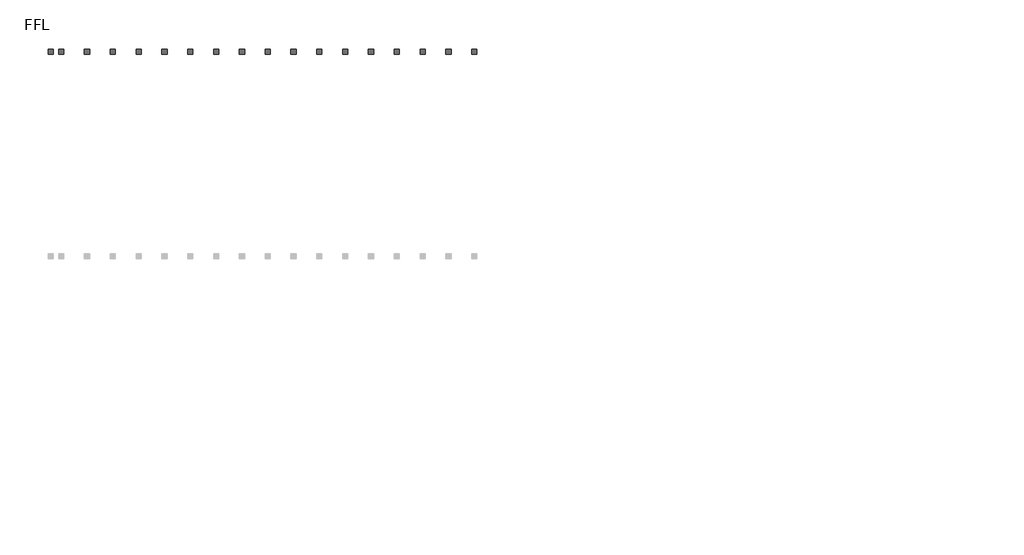
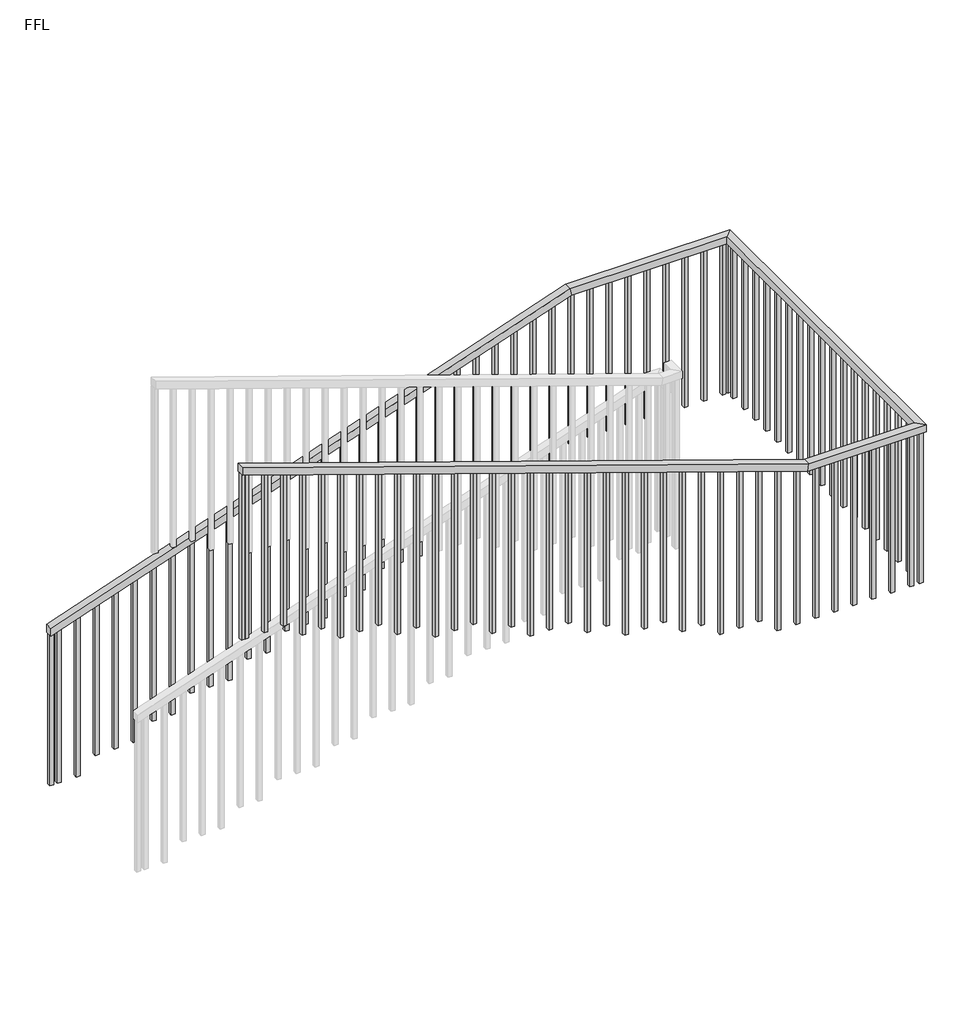
# One storey, part 2 of 2: 1 railing.
"""IFC4 building model written with IfcOpenShell, lengths in millimetres."""

from ifc_helpers import new_model, si_unit, frame, origin, place, context, project, spatial, polyline, outline, extrude, faceted_brep, element, save

model = new_model("IFC4")

# Units and contexts
model_context = context("Model", 3, world=origin())
ifc_project = project(units=[si_unit("LENGTHUNIT", "METRE", prefix="MILLI")], contexts=[model_context])

# Site, building, storey
site = spatial("IfcSite", under=ifc_project)
building = spatial("IfcBuilding", under=site)
storey = spatial("IfcBuildingStorey", under=building, Name="FFL", Elevation=3000.0)

# Railing
placement = place(None, origin())
element("IfcRailing", 1, ObjectType="1100mm", at=placement, inside=storey, context=model_context, shape_type="SolidModel", body=[
    faceted_brep([(-40149.9681829, 17835.7234223, 4656.2088216), (-40149.9681829, 17835.7234223, 4603.3636913), (-40149.9681829, 17785.7234223, 4603.3636913), (-40149.9681829, 17785.7234223, 4656.2088216), (-36733.6681829, 17835.7234223, 5824.9785156), (-36725.3519007, 17835.7234223, 5774.9785156), (-36725.3519007, 17785.7234223, 5774.9785156), (-36733.6681829, 17785.7234223, 5824.9785156), (-35651.74796, 17835.7234223, 5824.9785156), (-35651.74796, 17835.7234223, 5774.9785156), (-35701.74796, 17785.7234223, 5774.9785156), (-35701.74796, 17785.7234223, 5824.9785156), (-35651.74796, 15601.3234223, 5824.9785156), (-35651.74796, 15601.3234223, 5774.9785156), (-35701.74796, 15651.3234223, 5774.9785156), (-35701.74796, 15651.3234223, 5824.9785156), (-36423.0954556, 15601.3234223, 5824.9785156), (-36431.4117378, 15601.3234223, 5774.9785156), (-36431.4117378, 15651.3234223, 5774.9785156), (-36423.0954556, 15651.3234223, 5824.9785156), (-40149.9681829, 15601.3234223, 7100.0), (-40149.9681829, 15651.3234223, 7100.0), (-40149.9681829, 15651.3234223, 7047.1548697), (-40149.9681829, 15601.3234223, 7047.1548697)], [[[0, 1, 2, 3]], [[1, 0, 4, 5]], [[2, 1, 5, 6]], [[3, 2, 6, 7]], [[0, 3, 7, 4]], [[5, 4, 8, 9]], [[6, 5, 9, 10]], [[7, 6, 10, 11]], [[4, 7, 11, 8]], [[9, 8, 12, 13]], [[10, 9, 13, 14]], [[11, 10, 14, 15]], [[8, 11, 15, 12]], [[13, 12, 16, 17]], [[14, 13, 17, 18]], [[15, 14, 18, 19]], [[12, 15, 19, 16]], [[20, 21, 22, 23]], [[17, 16, 20, 23]], [[18, 17, 23, 22]], [[19, 18, 22, 21]], [[16, 19, 21, 20]]]),
    extrude(outline(polyline([(7030.6579768, -40101.74796), (7039.2108681, -40126.74796), (5893.7482096, -40126.74796), (5893.7482096, -40101.74796), (7030.6579768, -40101.74796)])), frame((0.0, 15613.8234223, 0.0), z_axis=(0.0, 1.0, 0.0), x_axis=(0.0, 0.0, 1.0)), (0.0, 0.0, 1.0), 25.0),
    extrude(outline(polyline([(6987.8935206, -39976.74796), (6996.4464119, -40001.74796), (5893.7482096, -40001.74796), (5893.7482096, -39976.74796), (6987.8935206, -39976.74796)])), frame((0.0, 15613.8234223, 0.0), z_axis=(0.0, 1.0, 0.0), x_axis=(0.0, 0.0, 1.0)), (0.0, 0.0, 1.0), 25.0),
    extrude(outline(polyline([(6945.1290644, -39851.74796), (6953.6819557, -39876.74796), (5893.7482096, -39876.74796), (5893.7482096, -39851.74796), (6945.1290644, -39851.74796)])), frame((0.0, 15613.8234223, 0.0), z_axis=(0.0, 1.0, 0.0), x_axis=(0.0, 0.0, 1.0)), (0.0, 0.0, 1.0), 25.0),
    extrude(outline(polyline([(6902.3646082, -39726.74796), (6910.9174995, -39751.74796), (5787.4964193, -39751.74796), (5787.4964193, -39726.74796), (6902.3646082, -39726.74796)])), frame((0.0, 15613.8234223, 0.0), z_axis=(0.0, 1.0, 0.0), x_axis=(0.0, 0.0, 1.0)), (0.0, 0.0, 1.0), 25.0),
    extrude(outline(polyline([(6859.600152, -39601.74796), (6868.1530432, -39626.74796), (5787.4964193, -39626.74796), (5787.4964193, -39601.74796), (6859.600152, -39601.74796)])), frame((0.0, 15613.8234223, 0.0), z_axis=(0.0, 1.0, 0.0), x_axis=(0.0, 0.0, 1.0)), (0.0, 0.0, 1.0), 25.0),
    extrude(outline(polyline([(6816.8356958, -39476.74796), (6825.388587, -39501.74796), (5681.2446289, -39501.74796), (5681.2446289, -39476.74796), (6816.8356958, -39476.74796)])), frame((0.0, 15613.8234223, 0.0), z_axis=(0.0, 1.0, 0.0), x_axis=(0.0, 0.0, 1.0)), (0.0, 0.0, 1.0), 25.0),
    extrude(outline(polyline([(6774.0712396, -39351.74796), (6782.6241308, -39376.74796), (5681.2446289, -39376.74796), (5681.2446289, -39351.74796), (6774.0712396, -39351.74796)])), frame((0.0, 15613.8234223, 0.0), z_axis=(0.0, 1.0, 0.0), x_axis=(0.0, 0.0, 1.0)), (0.0, 0.0, 1.0), 25.0),
    extrude(outline(polyline([(6731.3067834, -39226.74796), (6739.8596746, -39251.74796), (5681.2446289, -39251.74796), (5681.2446289, -39226.74796), (6731.3067834, -39226.74796)])), frame((0.0, 15613.8234223, 0.0), z_axis=(0.0, 1.0, 0.0), x_axis=(0.0, 0.0, 1.0)), (0.0, 0.0, 1.0), 25.0),
    extrude(outline(polyline([(6688.6114486, -39101.74796), (6697.1643398, -39126.74796), (5574.9928385, -39126.74796), (5574.9928385, -39101.74796), (6688.6114486, -39101.74796)])), frame((0.0, 15613.8234223, 0.0), z_axis=(0.0, 1.0, 0.0), x_axis=(0.0, 0.0, 1.0)), (0.0, 0.0, 1.0), 25.0),
    extrude(outline(polyline([(6645.8469924, -38976.74796), (6654.3998836, -39001.74796), (5574.9928385, -39001.74796), (5574.9928385, -38976.74796), (6645.8469924, -38976.74796)])), frame((0.0, 15613.8234223, 0.0), z_axis=(0.0, 1.0, 0.0), x_axis=(0.0, 0.0, 1.0)), (0.0, 0.0, 1.0), 25.0),
    extrude(outline(polyline([(6603.0825361, -38851.74796), (6611.6354274, -38876.74796), (5468.7410482, -38876.74796), (5468.7410482, -38851.74796), (6603.0825361, -38851.74796)])), frame((0.0, 15613.8234223, 0.0), z_axis=(0.0, 1.0, 0.0), x_axis=(0.0, 0.0, 1.0)), (0.0, 0.0, 1.0), 25.0),
    extrude(outline(polyline([(6560.3180799, -38726.74796), (6568.8709712, -38751.74796), (5468.7410482, -38751.74796), (5468.7410482, -38726.74796), (6560.3180799, -38726.74796)])), frame((0.0, 15613.8234223, 0.0), z_axis=(0.0, 1.0, 0.0), x_axis=(0.0, 0.0, 1.0)), (0.0, 0.0, 1.0), 25.0),
    extrude(outline(polyline([(6517.5536237, -38601.74796), (6526.106515, -38626.74796), (5468.7410482, -38626.74796), (5468.7410482, -38601.74796), (6517.5536237, -38601.74796)])), frame((0.0, 15613.8234223, 0.0), z_axis=(0.0, 1.0, 0.0), x_axis=(0.0, 0.0, 1.0)), (0.0, 0.0, 1.0), 25.0),
    extrude(outline(polyline([(6474.7891675, -38476.74796), (6483.3420588, -38501.74796), (5362.4892578, -38501.74796), (5362.4892578, -38476.74796), (6474.7891675, -38476.74796)])), frame((0.0, 15613.8234223, 0.0), z_axis=(0.0, 1.0, 0.0), x_axis=(0.0, 0.0, 1.0)), (0.0, 0.0, 1.0), 25.0),
    extrude(outline(polyline([(6432.0247113, -38351.74796), (6440.5776025, -38376.74796), (5362.4892578, -38376.74796), (5362.4892578, -38351.74796), (6432.0247113, -38351.74796)])), frame((0.0, 15613.8234223, 0.0), z_axis=(0.0, 1.0, 0.0), x_axis=(0.0, 0.0, 1.0)), (0.0, 0.0, 1.0), 25.0),
    extrude(outline(polyline([(6389.2602551, -38226.74796), (6397.8131463, -38251.74796), (5256.2374674, -38251.74796), (5256.2374674, -38226.74796), (6389.2602551, -38226.74796)])), frame((0.0, 15613.8234223, 0.0), z_axis=(0.0, 1.0, 0.0), x_axis=(0.0, 0.0, 1.0)), (0.0, 0.0, 1.0), 25.0),
    extrude(outline(polyline([(6346.4957989, -38101.74796), (6355.0486901, -38126.74796), (5256.2374674, -38126.74796), (5256.2374674, -38101.74796), (6346.4957989, -38101.74796)])), frame((0.0, 15613.8234223, 0.0), z_axis=(0.0, 1.0, 0.0), x_axis=(0.0, 0.0, 1.0)), (0.0, 0.0, 1.0), 25.0),
    extrude(outline(polyline([(6303.7313427, -37976.74796), (6312.2842339, -38001.74796), (5256.2374674, -38001.74796), (5256.2374674, -37976.74796), (6303.7313427, -37976.74796)])), frame((0.0, 15613.8234223, 0.0), z_axis=(0.0, 1.0, 0.0), x_axis=(0.0, 0.0, 1.0)), (0.0, 0.0, 1.0), 25.0),
    extrude(outline(polyline([(6260.9668865, -37851.74796), (6269.5197777, -37876.74796), (5149.9856771, -37876.74796), (5149.9856771, -37851.74796), (6260.9668865, -37851.74796)])), frame((0.0, 15613.8234223, 0.0), z_axis=(0.0, 1.0, 0.0), x_axis=(0.0, 0.0, 1.0)), (0.0, 0.0, 1.0), 25.0),
    extrude(outline(polyline([(6218.2024303, -37726.74796), (6226.7553215, -37751.74796), (5149.9856771, -37751.74796), (5149.9856771, -37726.74796), (6218.2024303, -37726.74796)])), frame((0.0, 15613.8234223, 0.0), z_axis=(0.0, 1.0, 0.0), x_axis=(0.0, 0.0, 1.0)), (0.0, 0.0, 1.0), 25.0),
    extrude(outline(polyline([(6175.437974, -37601.74796), (6183.9908653, -37626.74796), (5043.7338867, -37626.74796), (5043.7338867, -37601.74796), (6175.437974, -37601.74796)])), frame((0.0, 15613.8234223, 0.0), z_axis=(0.0, 1.0, 0.0), x_axis=(0.0, 0.0, 1.0)), (0.0, 0.0, 1.0), 25.0),
    extrude(outline(polyline([(6132.6735178, -37476.74796), (6141.2264091, -37501.74796), (5043.7338867, -37501.74796), (5043.7338867, -37476.74796), (6132.6735178, -37476.74796)])), frame((0.0, 15613.8234223, 0.0), z_axis=(0.0, 1.0, 0.0), x_axis=(0.0, 0.0, 1.0)), (0.0, 0.0, 1.0), 25.0),
    extrude(outline(polyline([(6089.9090616, -37351.74796), (6098.4619529, -37376.74796), (5043.7338867, -37376.74796), (5043.7338867, -37351.74796), (6089.9090616, -37351.74796)])), frame((0.0, 15613.8234223, 0.0), z_axis=(0.0, 1.0, 0.0), x_axis=(0.0, 0.0, 1.0)), (0.0, 0.0, 1.0), 25.0),
    extrude(outline(polyline([(6047.1446054, -37226.74796), (6055.6974967, -37251.74796), (4937.4820964, -37251.74796), (4937.4820964, -37226.74796), (6047.1446054, -37226.74796)])), frame((0.0, 15613.8234223, 0.0), z_axis=(0.0, 1.0, 0.0), x_axis=(0.0, 0.0, 1.0)), (0.0, 0.0, 1.0), 25.0),
    extrude(outline(polyline([(6004.3801492, -37101.74796), (6012.9330404, -37126.74796), (4937.4820964, -37126.74796), (4937.4820964, -37101.74796), (6004.3801492, -37101.74796)])), frame((0.0, 15613.8234223, 0.0), z_axis=(0.0, 1.0, 0.0), x_axis=(0.0, 0.0, 1.0)), (0.0, 0.0, 1.0), 25.0),
    extrude(outline(polyline([(5961.615693, -36976.74796), (5970.1685842, -37001.74796), (4831.230306, -37001.74796), (4831.230306, -36976.74796), (5961.615693, -36976.74796)])), frame((0.0, 15613.8234223, 0.0), z_axis=(0.0, 1.0, 0.0), x_axis=(0.0, 0.0, 1.0)), (0.0, 0.0, 1.0), 25.0),
    extrude(outline(polyline([(5918.8512368, -36851.74796), (5927.404128, -36876.74796), (4831.230306, -36876.74796), (4831.230306, -36851.74796), (5918.8512368, -36851.74796)])), frame((0.0, 15613.8234223, 0.0), z_axis=(0.0, 1.0, 0.0), x_axis=(0.0, 0.0, 1.0)), (0.0, 0.0, 1.0), 25.0),
    extrude(outline(polyline([(5876.0867806, -36726.74796), (5884.6396718, -36751.74796), (4831.230306, -36751.74796), (4831.230306, -36726.74796), (5876.0867806, -36726.74796)])), frame((0.0, 15613.8234223, 0.0), z_axis=(0.0, 1.0, 0.0), x_axis=(0.0, 0.0, 1.0)), (0.0, 0.0, 1.0), 25.0),
    extrude(outline(polyline([(5833.3223244, -36601.74796), (5841.8752156, -36626.74796), (4724.9785156, -36626.74796), (4724.9785156, -36601.74796), (5833.3223244, -36601.74796)])), frame((0.0, 15613.8234223, 0.0), z_axis=(0.0, 1.0, 0.0), x_axis=(0.0, 0.0, 1.0)), (0.0, 0.0, 1.0), 25.0),
    extrude(outline(polyline([(5790.5578682, -36476.74796), (5799.1107594, -36501.74796), (4724.9785156, -36501.74796), (4724.9785156, -36476.74796), (5790.5578682, -36476.74796)])), frame((0.0, 15613.8234223, 0.0), z_axis=(0.0, 1.0, 0.0), x_axis=(0.0, 0.0, 1.0)), (0.0, 0.0, 1.0), 25.0),
    extrude(outline(polyline([(-36351.74796, 15613.8234223), (-36376.74796, 15613.8234223), (-36376.74796, 15638.8234223), (-36351.74796, 15638.8234223), (-36351.74796, 15613.8234223)])), frame((0.0, 0.0, 4724.9785156), z_axis=(0.0, 0.0, 1.0), x_axis=(1.0, 0.0, 0.0)), (0.0, 0.0, 1.0), 1050.0),
    extrude(outline(polyline([(-36226.74796, 15613.8234223), (-36251.74796, 15613.8234223), (-36251.74796, 15638.8234223), (-36226.74796, 15638.8234223), (-36226.74796, 15613.8234223)])), frame((0.0, 0.0, 4724.9785156), z_axis=(0.0, 0.0, 1.0), x_axis=(1.0, 0.0, 0.0)), (0.0, 0.0, 1.0), 1050.0),
    extrude(outline(polyline([(-36101.74796, 15613.8234223), (-36126.74796, 15613.8234223), (-36126.74796, 15638.8234223), (-36101.74796, 15638.8234223), (-36101.74796, 15613.8234223)])), frame((0.0, 0.0, 4724.9785156), z_axis=(0.0, 0.0, 1.0), x_axis=(1.0, 0.0, 0.0)), (0.0, 0.0, 1.0), 1050.0),
    extrude(outline(polyline([(-35976.74796, 15613.8234223), (-36001.74796, 15613.8234223), (-36001.74796, 15638.8234223), (-35976.74796, 15638.8234223), (-35976.74796, 15613.8234223)])), frame((0.0, 0.0, 4724.9785156), z_axis=(0.0, 0.0, 1.0), x_axis=(1.0, 0.0, 0.0)), (0.0, 0.0, 1.0), 1050.0),
    extrude(outline(polyline([(-35851.74796, 15613.8234223), (-35876.74796, 15613.8234223), (-35876.74796, 15638.8234223), (-35851.74796, 15638.8234223), (-35851.74796, 15613.8234223)])), frame((0.0, 0.0, 4724.9785156), z_axis=(0.0, 0.0, 1.0), x_axis=(1.0, 0.0, 0.0)), (0.0, 0.0, 1.0), 1050.0),
    extrude(outline(polyline([(-35726.74796, 15613.8234223), (-35751.74796, 15613.8234223), (-35751.74796, 15638.8234223), (-35726.74796, 15638.8234223), (-35726.74796, 15613.8234223)])), frame((0.0, 0.0, 4724.9785156), z_axis=(0.0, 0.0, 1.0), x_axis=(1.0, 0.0, 0.0)), (0.0, 0.0, 1.0), 1050.0),
    extrude(outline(polyline([(-35664.24796, 15760.7234223), (-35664.24796, 15735.7234223), (-35689.24796, 15735.7234223), (-35689.24796, 15760.7234223), (-35664.24796, 15760.7234223)])), frame((0.0, 0.0, 4724.9785156), z_axis=(0.0, 0.0, 1.0), x_axis=(1.0, 0.0, 0.0)), (0.0, 0.0, 1.0), 1050.0),
    extrude(outline(polyline([(-35664.24796, 15885.7234223), (-35664.24796, 15860.7234223), (-35689.24796, 15860.7234223), (-35689.24796, 15885.7234223), (-35664.24796, 15885.7234223)])), frame((0.0, 0.0, 4724.9785156), z_axis=(0.0, 0.0, 1.0), x_axis=(1.0, 0.0, 0.0)), (0.0, 0.0, 1.0), 1050.0),
    extrude(outline(polyline([(-35664.24796, 16010.7234223), (-35664.24796, 15985.7234223), (-35689.24796, 15985.7234223), (-35689.24796, 16010.7234223), (-35664.24796, 16010.7234223)])), frame((0.0, 0.0, 4724.9785156), z_axis=(0.0, 0.0, 1.0), x_axis=(1.0, 0.0, 0.0)), (0.0, 0.0, 1.0), 1050.0),
    extrude(outline(polyline([(-35664.24796, 16135.7234223), (-35664.24796, 16110.7234223), (-35689.24796, 16110.7234223), (-35689.24796, 16135.7234223), (-35664.24796, 16135.7234223)])), frame((0.0, 0.0, 4724.9785156), z_axis=(0.0, 0.0, 1.0), x_axis=(1.0, 0.0, 0.0)), (0.0, 0.0, 1.0), 1050.0),
    extrude(outline(polyline([(-35664.24796, 16260.7234223), (-35664.24796, 16235.7234223), (-35689.24796, 16235.7234223), (-35689.24796, 16260.7234223), (-35664.24796, 16260.7234223)])), frame((0.0, 0.0, 4724.9785156), z_axis=(0.0, 0.0, 1.0), x_axis=(1.0, 0.0, 0.0)), (0.0, 0.0, 1.0), 1050.0),
    extrude(outline(polyline([(-35664.24796, 16385.7234223), (-35664.24796, 16360.7234223), (-35689.24796, 16360.7234223), (-35689.24796, 16385.7234223), (-35664.24796, 16385.7234223)])), frame((0.0, 0.0, 4724.9785156), z_axis=(0.0, 0.0, 1.0), x_axis=(1.0, 0.0, 0.0)), (0.0, 0.0, 1.0), 1050.0),
    extrude(outline(polyline([(-35664.24796, 16510.7234223), (-35664.24796, 16485.7234223), (-35689.24796, 16485.7234223), (-35689.24796, 16510.7234223), (-35664.24796, 16510.7234223)])), frame((0.0, 0.0, 4724.9785156), z_axis=(0.0, 0.0, 1.0), x_axis=(1.0, 0.0, 0.0)), (0.0, 0.0, 1.0), 1050.0),
    extrude(outline(polyline([(-35664.24796, 16635.7234223), (-35664.24796, 16610.7234223), (-35689.24796, 16610.7234223), (-35689.24796, 16635.7234223), (-35664.24796, 16635.7234223)])), frame((0.0, 0.0, 4724.9785156), z_axis=(0.0, 0.0, 1.0), x_axis=(1.0, 0.0, 0.0)), (0.0, 0.0, 1.0), 1050.0),
    extrude(outline(polyline([(-35664.24796, 16760.7234223), (-35664.24796, 16735.7234223), (-35689.24796, 16735.7234223), (-35689.24796, 16760.7234223), (-35664.24796, 16760.7234223)])), frame((0.0, 0.0, 4724.9785156), z_axis=(0.0, 0.0, 1.0), x_axis=(1.0, 0.0, 0.0)), (0.0, 0.0, 1.0), 1050.0),
    extrude(outline(polyline([(-35664.24796, 16885.7234223), (-35664.24796, 16860.7234223), (-35689.24796, 16860.7234223), (-35689.24796, 16885.7234223), (-35664.24796, 16885.7234223)])), frame((0.0, 0.0, 4724.9785156), z_axis=(0.0, 0.0, 1.0), x_axis=(1.0, 0.0, 0.0)), (0.0, 0.0, 1.0), 1050.0),
    extrude(outline(polyline([(-35664.24796, 17010.7234223), (-35664.24796, 16985.7234223), (-35689.24796, 16985.7234223), (-35689.24796, 17010.7234223), (-35664.24796, 17010.7234223)])), frame((0.0, 0.0, 4724.9785156), z_axis=(0.0, 0.0, 1.0), x_axis=(1.0, 0.0, 0.0)), (0.0, 0.0, 1.0), 1050.0),
    extrude(outline(polyline([(-35664.24796, 17135.7234223), (-35664.24796, 17110.7234223), (-35689.24796, 17110.7234223), (-35689.24796, 17135.7234223), (-35664.24796, 17135.7234223)])), frame((0.0, 0.0, 4724.9785156), z_axis=(0.0, 0.0, 1.0), x_axis=(1.0, 0.0, 0.0)), (0.0, 0.0, 1.0), 1050.0),
    extrude(outline(polyline([(-35664.24796, 17260.7234223), (-35664.24796, 17235.7234223), (-35689.24796, 17235.7234223), (-35689.24796, 17260.7234223), (-35664.24796, 17260.7234223)])), frame((0.0, 0.0, 4724.9785156), z_axis=(0.0, 0.0, 1.0), x_axis=(1.0, 0.0, 0.0)), (0.0, 0.0, 1.0), 1050.0),
    extrude(outline(polyline([(-35664.24796, 17385.7234223), (-35664.24796, 17360.7234223), (-35689.24796, 17360.7234223), (-35689.24796, 17385.7234223), (-35664.24796, 17385.7234223)])), frame((0.0, 0.0, 4724.9785156), z_axis=(0.0, 0.0, 1.0), x_axis=(1.0, 0.0, 0.0)), (0.0, 0.0, 1.0), 1050.0),
    extrude(outline(polyline([(-35664.24796, 17510.7234223), (-35664.24796, 17485.7234223), (-35689.24796, 17485.7234223), (-35689.24796, 17510.7234223), (-35664.24796, 17510.7234223)])), frame((0.0, 0.0, 4724.9785156), z_axis=(0.0, 0.0, 1.0), x_axis=(1.0, 0.0, 0.0)), (0.0, 0.0, 1.0), 1050.0),
    extrude(outline(polyline([(-35664.24796, 17635.7234223), (-35664.24796, 17610.7234223), (-35689.24796, 17610.7234223), (-35689.24796, 17635.7234223), (-35664.24796, 17635.7234223)])), frame((0.0, 0.0, 4724.9785156), z_axis=(0.0, 0.0, 1.0), x_axis=(1.0, 0.0, 0.0)), (0.0, 0.0, 1.0), 1050.0),
    extrude(outline(polyline([(-35664.24796, 17760.7234223), (-35664.24796, 17735.7234223), (-35689.24796, 17735.7234223), (-35689.24796, 17760.7234223), (-35664.24796, 17760.7234223)])), frame((0.0, 0.0, 4724.9785156), z_axis=(0.0, 0.0, 1.0), x_axis=(1.0, 0.0, 0.0)), (0.0, 0.0, 1.0), 1050.0),
    extrude(outline(polyline([(-35724.9681829, 17823.2234223), (-35699.9681829, 17823.2234223), (-35699.9681829, 17798.2234223), (-35724.9681829, 17798.2234223), (-35724.9681829, 17823.2234223)])), frame((0.0, 0.0, 4724.9785156), z_axis=(0.0, 0.0, 1.0), x_axis=(1.0, 0.0, 0.0)), (0.0, 0.0, 1.0), 1050.0),
    extrude(outline(polyline([(-35849.9681829, 17823.2234223), (-35824.9681829, 17823.2234223), (-35824.9681829, 17798.2234223), (-35849.9681829, 17798.2234223), (-35849.9681829, 17823.2234223)])), frame((0.0, 0.0, 4724.9785156), z_axis=(0.0, 0.0, 1.0), x_axis=(1.0, 0.0, 0.0)), (0.0, 0.0, 1.0), 1050.0),
    extrude(outline(polyline([(-35974.9681829, 17823.2234223), (-35949.9681829, 17823.2234223), (-35949.9681829, 17798.2234223), (-35974.9681829, 17798.2234223), (-35974.9681829, 17823.2234223)])), frame((0.0, 0.0, 4724.9785156), z_axis=(0.0, 0.0, 1.0), x_axis=(1.0, 0.0, 0.0)), (0.0, 0.0, 1.0), 1050.0),
    extrude(outline(polyline([(-36099.9681829, 17823.2234223), (-36074.9681829, 17823.2234223), (-36074.9681829, 17798.2234223), (-36099.9681829, 17798.2234223), (-36099.9681829, 17823.2234223)])), frame((0.0, 0.0, 4724.9785156), z_axis=(0.0, 0.0, 1.0), x_axis=(1.0, 0.0, 0.0)), (0.0, 0.0, 1.0), 1050.0),
    extrude(outline(polyline([(-36224.9681829, 17823.2234223), (-36199.9681829, 17823.2234223), (-36199.9681829, 17798.2234223), (-36224.9681829, 17798.2234223), (-36224.9681829, 17823.2234223)])), frame((0.0, 0.0, 4724.9785156), z_axis=(0.0, 0.0, 1.0), x_axis=(1.0, 0.0, 0.0)), (0.0, 0.0, 1.0), 1050.0),
    extrude(outline(polyline([(-36349.9681829, 17823.2234223), (-36324.9681829, 17823.2234223), (-36324.9681829, 17798.2234223), (-36349.9681829, 17798.2234223), (-36349.9681829, 17823.2234223)])), frame((0.0, 0.0, 4724.9785156), z_axis=(0.0, 0.0, 1.0), x_axis=(1.0, 0.0, 0.0)), (0.0, 0.0, 1.0), 1050.0),
    extrude(outline(polyline([(-36474.9681829, 17823.2234223), (-36449.9681829, 17823.2234223), (-36449.9681829, 17798.2234223), (-36474.9681829, 17798.2234223), (-36474.9681829, 17823.2234223)])), frame((0.0, 0.0, 4724.9785156), z_axis=(0.0, 0.0, 1.0), x_axis=(1.0, 0.0, 0.0)), (0.0, 0.0, 1.0), 1050.0),
    extrude(outline(polyline([(-36599.9681829, 17823.2234223), (-36574.9681829, 17823.2234223), (-36574.9681829, 17798.2234223), (-36599.9681829, 17798.2234223), (-36599.9681829, 17823.2234223)])), frame((0.0, 0.0, 4724.9785156), z_axis=(0.0, 0.0, 1.0), x_axis=(1.0, 0.0, 0.0)), (0.0, 0.0, 1.0), 1050.0),
    extrude(outline(polyline([(-36724.9681829, 17823.2234223), (-36699.9681829, 17823.2234223), (-36699.9681829, 17798.2234223), (-36724.9681829, 17798.2234223), (-36724.9681829, 17823.2234223)])), frame((0.0, 0.0, 4724.9785156), z_axis=(0.0, 0.0, 1.0), x_axis=(1.0, 0.0, 0.0)), (0.0, 0.0, 1.0), 1050.0),
    extrude(outline(polyline([(4618.7267253, -36849.9681829), (4618.7267253, -36824.9681829), (5740.8982265, -36824.9681829), (5732.3453353, -36849.9681829), (4618.7267253, -36849.9681829)])), frame((0.0, 17798.2234223, 0.0), z_axis=(0.0, 1.0, 0.0), x_axis=(0.0, 0.0, 1.0)), (0.0, 0.0, 1.0), 25.0),
    extrude(outline(polyline([(4618.7267253, -36974.9681829), (4618.7267253, -36949.9681829), (5698.1337703, -36949.9681829), (5689.5808791, -36974.9681829), (4618.7267253, -36974.9681829)])), frame((0.0, 17798.2234223, 0.0), z_axis=(0.0, 1.0, 0.0), x_axis=(0.0, 0.0, 1.0)), (0.0, 0.0, 1.0), 25.0),
    extrude(outline(polyline([(4512.4749349, -37099.9681829), (4512.4749349, -37074.9681829), (5655.3693141, -37074.9681829), (5646.8164229, -37099.9681829), (4512.4749349, -37099.9681829)])), frame((0.0, 17798.2234223, 0.0), z_axis=(0.0, 1.0, 0.0), x_axis=(0.0, 0.0, 1.0)), (0.0, 0.0, 1.0), 25.0),
    extrude(outline(polyline([(4512.4749349, -37224.9681829), (4512.4749349, -37199.9681829), (5612.6048579, -37199.9681829), (5604.0519667, -37224.9681829), (4512.4749349, -37224.9681829)])), frame((0.0, 17798.2234223, 0.0), z_axis=(0.0, 1.0, 0.0), x_axis=(0.0, 0.0, 1.0)), (0.0, 0.0, 1.0), 25.0),
    extrude(outline(polyline([(4512.4749349, -37349.9681829), (4512.4749349, -37324.9681829), (5569.8404017, -37324.9681829), (5561.2875104, -37349.9681829), (4512.4749349, -37349.9681829)])), frame((0.0, 17798.2234223, 0.0), z_axis=(0.0, 1.0, 0.0), x_axis=(0.0, 0.0, 1.0)), (0.0, 0.0, 1.0), 25.0),
    extrude(outline(polyline([(4406.2231445, -37474.9681829), (4406.2231445, -37449.9681829), (5527.0759455, -37449.9681829), (5518.5230542, -37474.9681829), (4406.2231445, -37474.9681829)])), frame((0.0, 17798.2234223, 0.0), z_axis=(0.0, 1.0, 0.0), x_axis=(0.0, 0.0, 1.0)), (0.0, 0.0, 1.0), 25.0),
    extrude(outline(polyline([(4406.2231445, -37599.9681829), (4406.2231445, -37574.9681829), (5484.3114893, -37574.9681829), (5475.758598, -37599.9681829), (4406.2231445, -37599.9681829)])), frame((0.0, 17798.2234223, 0.0), z_axis=(0.0, 1.0, 0.0), x_axis=(0.0, 0.0, 1.0)), (0.0, 0.0, 1.0), 25.0),
    extrude(outline(polyline([(4299.9713542, -37724.9681829), (4299.9713542, -37699.9681829), (5441.5470331, -37699.9681829), (5432.9941418, -37724.9681829), (4299.9713542, -37724.9681829)])), frame((0.0, 17798.2234223, 0.0), z_axis=(0.0, 1.0, 0.0), x_axis=(0.0, 0.0, 1.0)), (0.0, 0.0, 1.0), 25.0),
    extrude(outline(polyline([(4299.9713542, -37849.9681829), (4299.9713542, -37824.9681829), (5398.7825768, -37824.9681829), (5390.2296856, -37849.9681829), (4299.9713542, -37849.9681829)])), frame((0.0, 17798.2234223, 0.0), z_axis=(0.0, 1.0, 0.0), x_axis=(0.0, 0.0, 1.0)), (0.0, 0.0, 1.0), 25.0),
    extrude(outline(polyline([(4299.9713542, -37974.9681829), (4299.9713542, -37949.9681829), (5356.0181206, -37949.9681829), (5347.4652294, -37974.9681829), (4299.9713542, -37974.9681829)])), frame((0.0, 17798.2234223, 0.0), z_axis=(0.0, 1.0, 0.0), x_axis=(0.0, 0.0, 1.0)), (0.0, 0.0, 1.0), 25.0),
    extrude(outline(polyline([(4193.7195638, -38099.9681829), (4193.7195638, -38074.9681829), (5313.2536644, -38074.9681829), (5304.7007732, -38099.9681829), (4193.7195638, -38099.9681829)])), frame((0.0, 17798.2234223, 0.0), z_axis=(0.0, 1.0, 0.0), x_axis=(0.0, 0.0, 1.0)), (0.0, 0.0, 1.0), 25.0),
    extrude(outline(polyline([(4193.7195638, -38224.9681829), (4193.7195638, -38199.9681829), (5270.4892082, -38199.9681829), (5261.936317, -38224.9681829), (4193.7195638, -38224.9681829)])), frame((0.0, 17798.2234223, 0.0), z_axis=(0.0, 1.0, 0.0), x_axis=(0.0, 0.0, 1.0)), (0.0, 0.0, 1.0), 25.0),
    extrude(outline(polyline([(4087.4677734, -38349.9681829), (4087.4677734, -38324.9681829), (5227.724752, -38324.9681829), (5219.1718608, -38349.9681829), (4087.4677734, -38349.9681829)])), frame((0.0, 17798.2234223, 0.0), z_axis=(0.0, 1.0, 0.0), x_axis=(0.0, 0.0, 1.0)), (0.0, 0.0, 1.0), 25.0),
    extrude(outline(polyline([(4087.4677734, -38474.9681829), (4087.4677734, -38449.9681829), (5184.9602958, -38449.9681829), (5176.4074046, -38474.9681829), (4087.4677734, -38474.9681829)])), frame((0.0, 17798.2234223, 0.0), z_axis=(0.0, 1.0, 0.0), x_axis=(0.0, 0.0, 1.0)), (0.0, 0.0, 1.0), 25.0),
    extrude(outline(polyline([(4087.4677734, -38599.9681829), (4087.4677734, -38574.9681829), (5142.1958396, -38574.9681829), (5133.6429483, -38599.9681829), (4087.4677734, -38599.9681829)])), frame((0.0, 17798.2234223, 0.0), z_axis=(0.0, 1.0, 0.0), x_axis=(0.0, 0.0, 1.0)), (0.0, 0.0, 1.0), 25.0),
    extrude(outline(polyline([(3981.2159831, -38724.9681829), (3981.2159831, -38699.9681829), (5099.4313834, -38699.9681829), (5090.8784921, -38724.9681829), (3981.2159831, -38724.9681829)])), frame((0.0, 17798.2234223, 0.0), z_axis=(0.0, 1.0, 0.0), x_axis=(0.0, 0.0, 1.0)), (0.0, 0.0, 1.0), 25.0),
    extrude(outline(polyline([(3981.2159831, -38849.9681829), (3981.2159831, -38824.9681829), (5056.6669272, -38824.9681829), (5048.1140359, -38849.9681829), (3981.2159831, -38849.9681829)])), frame((0.0, 17798.2234223, 0.0), z_axis=(0.0, 1.0, 0.0), x_axis=(0.0, 0.0, 1.0)), (0.0, 0.0, 1.0), 25.0),
    extrude(outline(polyline([(3874.9641927, -38974.9681829), (3874.9641927, -38949.9681829), (5013.902471, -38949.9681829), (5005.3495797, -38974.9681829), (3874.9641927, -38974.9681829)])), frame((0.0, 17798.2234223, 0.0), z_axis=(0.0, 1.0, 0.0), x_axis=(0.0, 0.0, 1.0)), (0.0, 0.0, 1.0), 25.0),
    extrude(outline(polyline([(3874.9641927, -39099.9681829), (3874.9641927, -39074.9681829), (4971.1380147, -39074.9681829), (4962.5851235, -39099.9681829), (3874.9641927, -39099.9681829)])), frame((0.0, 17798.2234223, 0.0), z_axis=(0.0, 1.0, 0.0), x_axis=(0.0, 0.0, 1.0)), (0.0, 0.0, 1.0), 25.0),
    extrude(outline(polyline([(3874.9641927, -39224.9681829), (3874.9641927, -39199.9681829), (4928.3735585, -39199.9681829), (4919.8206673, -39224.9681829), (3874.9641927, -39224.9681829)])), frame((0.0, 17798.2234223, 0.0), z_axis=(0.0, 1.0, 0.0), x_axis=(0.0, 0.0, 1.0)), (0.0, 0.0, 1.0), 25.0),
    extrude(outline(polyline([(3768.7124023, -39349.9681829), (3768.7124023, -39324.9681829), (4885.6091023, -39324.9681829), (4877.0562111, -39349.9681829), (3768.7124023, -39349.9681829)])), frame((0.0, 17798.2234223, 0.0), z_axis=(0.0, 1.0, 0.0), x_axis=(0.0, 0.0, 1.0)), (0.0, 0.0, 1.0), 25.0),
    extrude(outline(polyline([(3768.7124023, -39474.9681829), (3768.7124023, -39449.9681829), (4842.8446461, -39449.9681829), (4834.2917549, -39474.9681829), (3768.7124023, -39474.9681829)])), frame((0.0, 17798.2234223, 0.0), z_axis=(0.0, 1.0, 0.0), x_axis=(0.0, 0.0, 1.0)), (0.0, 0.0, 1.0), 25.0),
    extrude(outline(polyline([(3662.460612, -39599.9681829), (3662.460612, -39574.9681829), (4800.0801899, -39574.9681829), (4791.5272987, -39599.9681829), (3662.460612, -39599.9681829)])), frame((0.0, 17798.2234223, 0.0), z_axis=(0.0, 1.0, 0.0), x_axis=(0.0, 0.0, 1.0)), (0.0, 0.0, 1.0), 25.0),
    extrude(outline(polyline([(3662.460612, -39724.9681829), (3662.460612, -39699.9681829), (4757.3157337, -39699.9681829), (4748.7628424, -39724.9681829), (3662.460612, -39724.9681829)])), frame((0.0, 17798.2234223, 0.0), z_axis=(0.0, 1.0, 0.0), x_axis=(0.0, 0.0, 1.0)), (0.0, 0.0, 1.0), 25.0),
    extrude(outline(polyline([(3662.460612, -39849.9681829), (3662.460612, -39824.9681829), (4714.5512775, -39824.9681829), (4705.9983862, -39849.9681829), (3662.460612, -39849.9681829)])), frame((0.0, 17798.2234223, 0.0), z_axis=(0.0, 1.0, 0.0), x_axis=(0.0, 0.0, 1.0)), (0.0, 0.0, 1.0), 25.0),
    extrude(outline(polyline([(3556.2088216, -39974.9681829), (3556.2088216, -39949.9681829), (4671.7868213, -39949.9681829), (4663.23393, -39974.9681829), (3556.2088216, -39974.9681829)])), frame((0.0, 17798.2234223, 0.0), z_axis=(0.0, 1.0, 0.0), x_axis=(0.0, 0.0, 1.0)), (0.0, 0.0, 1.0), 25.0),
    extrude(outline(polyline([(3556.2088216, -40099.9681829), (3556.2088216, -40074.9681829), (4629.0223651, -40074.9681829), (4620.4694738, -40099.9681829), (3556.2088216, -40099.9681829)])), frame((0.0, 17798.2234223, 0.0), z_axis=(0.0, 1.0, 0.0), x_axis=(0.0, 0.0, 1.0)), (0.0, 0.0, 1.0), 25.0),
    extrude(outline(polyline([(-35664.24796, 15638.8234223), (-35664.24796, 15613.8234223), (-35689.24796, 15613.8234223), (-35689.24796, 15638.8234223), (-35664.24796, 15638.8234223)])), frame((0.0, 0.0, 4724.9785156), z_axis=(0.0, 0.0, 1.0), x_axis=(1.0, 0.0, 0.0)), (0.0, 0.0, 1.0), 1050.0),
    extrude(outline(polyline([(-35689.24796, 17823.2234223), (-35664.24796, 17823.2234223), (-35664.24796, 17798.2234223), (-35689.24796, 17798.2234223), (-35689.24796, 17823.2234223)])), frame((0.0, 0.0, 4724.9785156), z_axis=(0.0, 0.0, 1.0), x_axis=(1.0, 0.0, 0.0)), (0.0, 0.0, 1.0), 1050.0),
    extrude(outline(polyline([(7038.6019785, -40124.9681829), (7047.1548697, -40149.9681829), (5893.7482096, -40149.9681829), (5893.7482096, -40124.9681829), (7038.6019785, -40124.9681829)])), frame((0.0, 15613.8234223, 0.0), z_axis=(0.0, 1.0, 0.0), x_axis=(0.0, 0.0, 1.0)), (0.0, 0.0, 1.0), 25.0),
    extrude(outline(polyline([(3556.2088216, -40149.9681829), (3556.2088216, -40124.9681829), (4611.9165826, -40124.9681829), (4603.3636913, -40149.9681829), (3556.2088216, -40149.9681829)])), frame((0.0, 17798.2234223, 0.0), z_axis=(0.0, 1.0, 0.0), x_axis=(0.0, 0.0, 1.0)), (0.0, 0.0, 1.0), 25.0),
])

save(model, "model.ifc")

# Revit data of these elements
# Type "1100mm"
#   built-in parameter 1008612 = 0.019685 (stored number, unit not read)
#   built-in parameter 1008611 = 0.019685 (stored number, unit not read)
#   built-in parameter 1008609 = 0.902231 (stored number, unit not read)
#   built-in parameter 1008604 = 0.19685 (stored number, unit not read)
#   built-in parameter 1008603 = 0.164042 (stored number, unit not read)
#   Railing Height = 3' - 7.30709"
#   built-in parameter 1008630 = 2
#   built-in parameter 1008610 = 2
#   built-in parameter 1008608 = 1
#   built-in parameter 1008618 = Baluster_Square : 25mm
# Element 1 (IfcRailing, "1100mm")
#   Phase Created = New Construction
